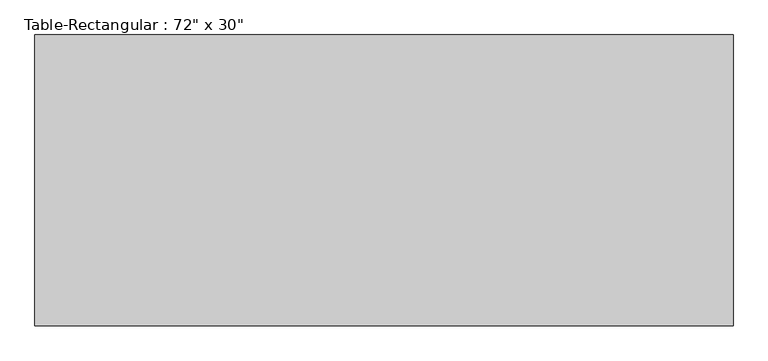
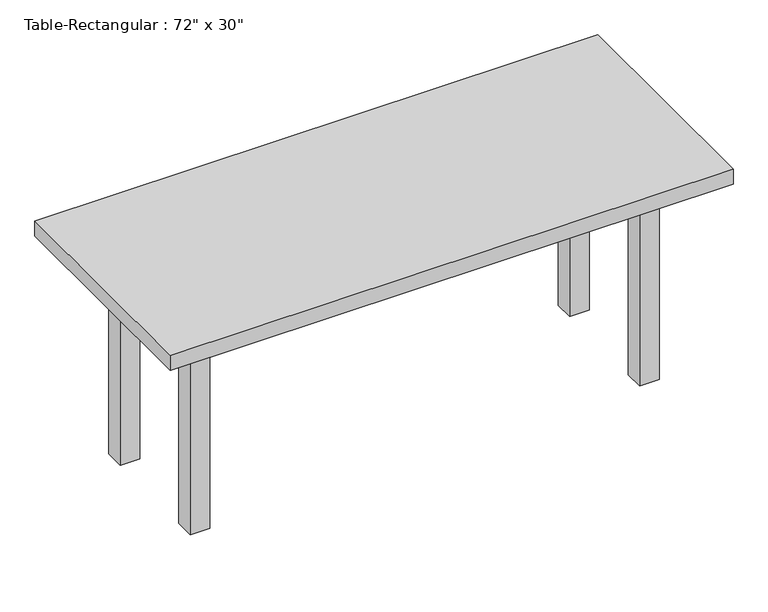
"""IFC4 building model written with IfcOpenShell, lengths in millimetres: furniture geometry."""

from ifc_helpers import new_model, si_unit, frame, origin, origin_with_axes, place, context, project, spatial, polyline, outline, extrude, source, transform, mapped, element, save


def furniture_03292632(model_context):
    return source(origin(), model_context, "Body", "SweptSolid", [
        extrude(outline(polyline([(-698.5, 228.6), (-698.5, 165.1), (-762.0, 165.1), (-762.0, 228.6), (-698.5, 228.6)])), origin_with_axes(), (0.0, 0.0, 1.0), 711.2),
        extrude(outline(polyline([(698.5, 228.6), (762.0, 228.6), (762.0, 165.1), (698.5, 165.1), (698.5, 228.6)])), origin_with_axes(), (0.0, 0.0, 1.0), 711.2),
        extrude(outline(polyline([(-698.5, -228.6), (-762.0, -228.6), (-762.0, -165.1), (-698.5, -165.1), (-698.5, -228.6)])), origin_with_axes(), (0.0, 0.0, 1.0), 711.2),
        extrude(outline(polyline([(698.5, -228.6), (698.5, -165.1), (762.0, -165.1), (762.0, -228.6), (698.5, -228.6)])), origin_with_axes(), (0.0, 0.0, 1.0), 711.2),
        extrude(outline(polyline([(914.4, 381.0), (914.4, -381.0), (-914.4, -381.0), (-914.4, 381.0), (914.4, 381.0)])), frame((0.0, 0.0, 711.2), z_axis=(0.0, 0.0, 1.0), x_axis=(1.0, 0.0, 0.0)), (0.0, 0.0, 1.0), 50.8),
        extrude(outline(polyline([(698.5, 190.5), (698.5, 165.1), (-698.5, 165.1), (-698.5, 190.5), (698.5, 190.5)])), frame((0.0, 0.0, 609.6), z_axis=(0.0, 0.0, 1.0), x_axis=(1.0, 0.0, 0.0)), (0.0, 0.0, 1.0), 101.6),
        extrude(outline(polyline([(698.5, -190.5), (-698.5, -190.5), (-698.5, -165.1), (698.5, -165.1), (698.5, -190.5)])), frame((0.0, 0.0, 609.6), z_axis=(0.0, 0.0, 1.0), x_axis=(1.0, 0.0, 0.0)), (0.0, 0.0, 1.0), 101.6),
        extrude(outline(polyline([(-711.2, -165.1), (-736.6, -165.1), (-736.6, 165.1), (-711.2, 165.1), (-711.2, -165.1)])), frame((0.0, 0.0, 609.6), z_axis=(0.0, 0.0, 1.0), x_axis=(1.0, 0.0, 0.0)), (0.0, 0.0, 1.0), 101.6),
        extrude(outline(polyline([(711.2, -165.1), (711.2, 165.1), (736.6, 165.1), (736.6, -165.1), (711.2, -165.1)])), frame((0.0, 0.0, 609.6), z_axis=(0.0, 0.0, 1.0), x_axis=(1.0, 0.0, 0.0)), (0.0, 0.0, 1.0), 101.6),
    ])


if __name__ == "__main__":
    model = new_model("IFC4")
    model_context = context("Model", 3, world=origin())
    ifc_project = project(units=[si_unit("LENGTHUNIT", "METRE", prefix="MILLI")], contexts=[model_context])
    site = spatial("IfcSite", under=ifc_project)
    building = spatial("IfcBuilding", under=site)
    placement = place(None, origin())
    furniture_shape = furniture_03292632(model_context)
    element("IfcFurniture", 1, ObjectType="Table-Rectangular : 72\" x 30\"", at=placement, inside=building, context=model_context, shape_type="MappedRepresentation", body=[
        mapped(furniture_shape, transform((0.0, 0.0, 0.0), x_axis=(1.0, 0.0, 0.0), y_axis=(0.0, 1.0, 0.0), z_axis=(0.0, 0.0, 1.0))),
    ])
    save(model, "model.ifc")

# Revit data of these elements
# Type "Table-Rectangular : 72\" x 30\""
#   Assembly Code = "E2020200"
#   Height = 2' - 6"
#   Length = 6' - 0"
#   Width = 2' - 6"
#   Base Material = Birch
#   Top Material = Birch
#   Default Elevation = 0
# Element 1 (IfcFurniture, "Table-Rectangular : 72\" x 30\"")
#   Materials on its faces: "Birch"
# Materials
#   "Birch": class "Wood", colour RGB 224 178 126, transparency 0, Description = "Betula Alleghaniensis", Cost = 0
